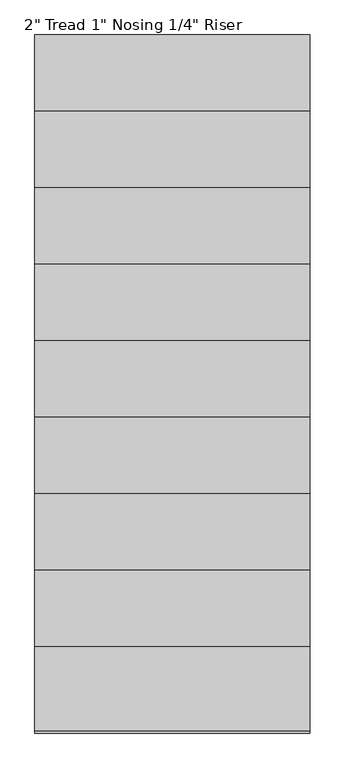
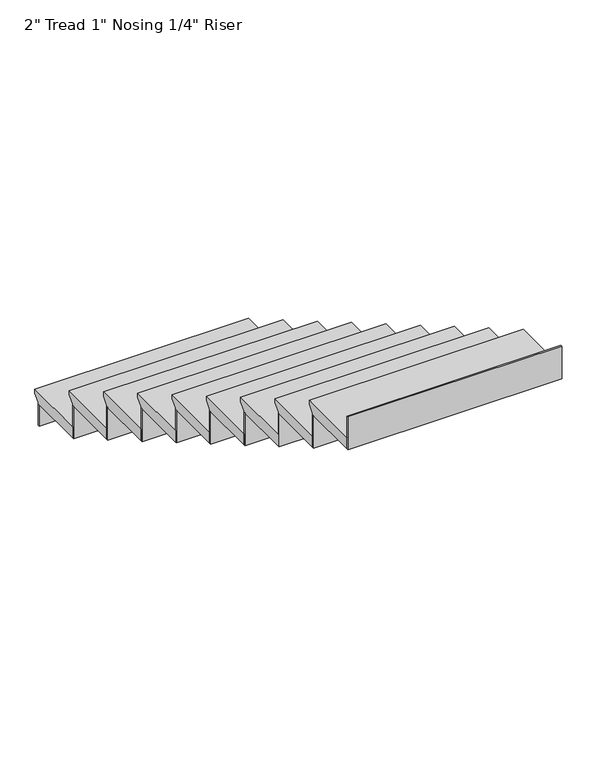
"""IFC4 building model written with IfcOpenShell, lengths in millimetres: stair flight geometry."""

from ifc_helpers import new_model, si_unit, origin, place, context, project, spatial, faceted_brep, source, transform, mapped, element, save


def stair_flight_05c21e37(model_context):
    return source(origin(), model_context, "Body", "Brep", [
        faceted_brep([(-4315.1137331, -4241.0593836, 6472.7714861), (-4315.1137331, -4241.0593836, 6491.8214861), (-3400.7137331, -4241.0593836, 6491.8214861), (-3400.7137331, -4241.0593836, 6472.7714861), (-4315.1137331, -4266.4593836, 6447.3714861), (-3400.7137331, -4266.4593836, 6447.3714861), (-4315.1137331, -4520.4593836, 6491.8214861), (-3400.7137331, -4520.4593836, 6491.8214861), (-3400.7137331, -4266.4593836, 6441.0214861), (-3400.7137331, -4520.4593836, 6441.0214861), (-4315.1137331, -4520.4593836, 6441.0214861), (-4315.1137331, -4266.4593836, 6441.0214861)], [[[0, 1, 2, 3]], [[4, 0, 3, 5]], [[2, 1, 6, 7]], [[8, 9, 10, 11]], [[2, 7, 9, 8, 5, 3]], [[8, 11, 4, 5]], [[6, 1, 0, 4, 11, 10]], [[7, 6, 10, 9]]]),
        faceted_brep([(-4315.1137331, -4266.4593836, 6441.0214861), (-4315.1137331, -4266.4593836, 6343.9725604), (-4315.1137331, -4272.8093836, 6343.9725604), (-4315.1137331, -4272.8093836, 6441.0214861), (-3400.7137331, -4266.4593836, 6441.0214861), (-3400.7137331, -4272.8093836, 6441.0214861), (-3400.7137331, -4272.8093836, 6343.9725604), (-3400.7137331, -4266.4593836, 6343.9725604)], [[[0, 1, 2, 3]], [[4, 5, 6, 7]], [[1, 0, 4, 7]], [[2, 1, 7, 6]], [[3, 2, 6, 5]], [[0, 3, 5, 4]]]),
        faceted_brep([(-4315.1137331, -4520.4593836, 6588.8704118), (-4315.1137331, -4520.4593836, 6441.0214861), (-4315.1137331, -4526.8093836, 6441.0214861), (-4315.1137331, -4526.8093836, 6588.8704118), (-3400.7137331, -4520.4593836, 6588.8704118), (-3400.7137331, -4526.8093836, 6588.8704118), (-3400.7137331, -4526.8093836, 6441.0214861), (-3400.7137331, -4520.4593836, 6441.0214861)], [[[0, 1, 2, 3]], [[4, 5, 6, 7]], [[1, 0, 4, 7]], [[2, 1, 7, 6]], [[3, 2, 6, 5]], [[0, 3, 5, 4]]]),
        faceted_brep([(-3400.7137331, -4495.0593836, 6639.6704118), (-4315.1137331, -4495.0593836, 6639.6704118), (-4315.1137331, -4774.4593836, 6639.6704118), (-3400.7137331, -4774.4593836, 6639.6704118), (-3400.7137331, -4520.4593836, 6588.8704118), (-3400.7137331, -4774.4593836, 6588.8704118), (-4315.1137331, -4774.4593836, 6588.8704118), (-4315.1137331, -4520.4593836, 6588.8704118), (-3400.7137331, -4520.4593836, 6595.2204118), (-3400.7137331, -4495.0593836, 6620.6204118), (-4315.1137331, -4520.4593836, 6595.2204118), (-4315.1137331, -4495.0593836, 6620.6204118)], [[[0, 1, 2, 3]], [[4, 5, 6, 7]], [[0, 3, 5, 4, 8, 9]], [[4, 7, 10, 8]], [[2, 1, 11, 10, 7, 6]], [[3, 2, 6, 5]], [[11, 1, 0, 9]], [[10, 11, 9, 8]]]),
        faceted_brep([(-4315.1137331, -4774.4593836, 6736.7193375), (-4315.1137331, -4774.4593836, 6588.8704118), (-4315.1137331, -4780.8093836, 6588.8704118), (-4315.1137331, -4780.8093836, 6736.7193375), (-3400.7137331, -4774.4593836, 6736.7193375), (-3400.7137331, -4780.8093836, 6736.7193375), (-3400.7137331, -4780.8093836, 6588.8704118), (-3400.7137331, -4774.4593836, 6588.8704118)], [[[0, 1, 2, 3]], [[4, 5, 6, 7]], [[1, 0, 4, 7]], [[2, 1, 7, 6]], [[3, 2, 6, 5]], [[0, 3, 5, 4]]]),
        faceted_brep([(-3400.7137331, -4749.0593836, 6787.5193375), (-4315.1137331, -4749.0593836, 6787.5193375), (-4315.1137331, -5028.4593836, 6787.5193375), (-3400.7137331, -5028.4593836, 6787.5193375), (-3400.7137331, -4774.4593836, 6736.7193375), (-3400.7137331, -5028.4593836, 6736.7193375), (-4315.1137331, -5028.4593836, 6736.7193375), (-4315.1137331, -4774.4593836, 6736.7193375), (-3400.7137331, -4774.4593836, 6743.0693375), (-3400.7137331, -4749.0593836, 6768.4693375), (-4315.1137331, -4774.4593836, 6743.0693375), (-4315.1137331, -4749.0593836, 6768.4693375)], [[[0, 1, 2, 3]], [[4, 5, 6, 7]], [[0, 3, 5, 4, 8, 9]], [[4, 7, 10, 8]], [[2, 1, 11, 10, 7, 6]], [[3, 2, 6, 5]], [[11, 1, 0, 9]], [[10, 11, 9, 8]]]),
        faceted_brep([(-4315.1137331, -5028.4593836, 6884.5682632), (-4315.1137331, -5028.4593836, 6736.7193375), (-4315.1137331, -5034.8093836, 6736.7193375), (-4315.1137331, -5034.8093836, 6884.5682632), (-3400.7137331, -5028.4593836, 6884.5682632), (-3400.7137331, -5034.8093836, 6884.5682632), (-3400.7137331, -5034.8093836, 6736.7193375), (-3400.7137331, -5028.4593836, 6736.7193375)], [[[0, 1, 2, 3]], [[4, 5, 6, 7]], [[1, 0, 4, 7]], [[2, 1, 7, 6]], [[3, 2, 6, 5]], [[0, 3, 5, 4]]]),
        faceted_brep([(-3400.7137331, -5003.0593836, 6935.3682632), (-4315.1137331, -5003.0593836, 6935.3682632), (-4315.1137331, -5282.4593836, 6935.3682632), (-3400.7137331, -5282.4593836, 6935.3682632), (-3400.7137331, -5028.4593836, 6884.5682632), (-3400.7137331, -5282.4593836, 6884.5682632), (-4315.1137331, -5282.4593836, 6884.5682632), (-4315.1137331, -5028.4593836, 6884.5682632), (-3400.7137331, -5028.4593836, 6890.9182632), (-3400.7137331, -5003.0593836, 6916.3182632), (-4315.1137331, -5028.4593836, 6890.9182632), (-4315.1137331, -5003.0593836, 6916.3182632)], [[[0, 1, 2, 3]], [[4, 5, 6, 7]], [[0, 3, 5, 4, 8, 9]], [[4, 7, 10, 8]], [[2, 1, 11, 10, 7, 6]], [[3, 2, 6, 5]], [[11, 1, 0, 9]], [[10, 11, 9, 8]]]),
        faceted_brep([(-4315.1137331, -5282.4593836, 7032.4171889), (-4315.1137331, -5282.4593836, 6884.5682632), (-4315.1137331, -5288.8093836, 6884.5682632), (-4315.1137331, -5288.8093836, 7032.4171889), (-3400.7137331, -5282.4593836, 7032.4171889), (-3400.7137331, -5288.8093836, 7032.4171889), (-3400.7137331, -5288.8093836, 6884.5682632), (-3400.7137331, -5282.4593836, 6884.5682632)], [[[0, 1, 2, 3]], [[4, 5, 6, 7]], [[1, 0, 4, 7]], [[2, 1, 7, 6]], [[3, 2, 6, 5]], [[0, 3, 5, 4]]]),
        faceted_brep([(-3400.7137331, -5257.0593836, 7083.2171889), (-4315.1137331, -5257.0593836, 7083.2171889), (-4315.1137331, -5536.4593836, 7083.2171889), (-3400.7137331, -5536.4593836, 7083.2171889), (-3400.7137331, -5282.4593836, 7032.4171889), (-3400.7137331, -5536.4593836, 7032.4171889), (-4315.1137331, -5536.4593836, 7032.4171889), (-4315.1137331, -5282.4593836, 7032.4171889), (-3400.7137331, -5282.4593836, 7038.7671889), (-3400.7137331, -5257.0593836, 7064.1671889), (-4315.1137331, -5282.4593836, 7038.7671889), (-4315.1137331, -5257.0593836, 7064.1671889)], [[[0, 1, 2, 3]], [[4, 5, 6, 7]], [[0, 3, 5, 4, 8, 9]], [[4, 7, 10, 8]], [[2, 1, 11, 10, 7, 6]], [[3, 2, 6, 5]], [[11, 1, 0, 9]], [[10, 11, 9, 8]]]),
        faceted_brep([(-4315.1137331, -5536.4593836, 7180.2661146), (-4315.1137331, -5536.4593836, 7032.4171889), (-4315.1137331, -5542.8093836, 7032.4171889), (-4315.1137331, -5542.8093836, 7180.2661146), (-3400.7137331, -5536.4593836, 7180.2661146), (-3400.7137331, -5542.8093836, 7180.2661146), (-3400.7137331, -5542.8093836, 7032.4171889), (-3400.7137331, -5536.4593836, 7032.4171889)], [[[0, 1, 2, 3]], [[4, 5, 6, 7]], [[1, 0, 4, 7]], [[2, 1, 7, 6]], [[3, 2, 6, 5]], [[0, 3, 5, 4]]]),
        faceted_brep([(-3400.7137331, -5511.0593836, 7231.0661146), (-4315.1137331, -5511.0593836, 7231.0661146), (-4315.1137331, -5790.4593836, 7231.0661146), (-3400.7137331, -5790.4593836, 7231.0661146), (-3400.7137331, -5536.4593836, 7180.2661146), (-3400.7137331, -5790.4593836, 7180.2661146), (-4315.1137331, -5790.4593836, 7180.2661146), (-4315.1137331, -5536.4593836, 7180.2661146), (-3400.7137331, -5536.4593836, 7186.6161146), (-3400.7137331, -5511.0593836, 7212.0161146), (-4315.1137331, -5536.4593836, 7186.6161146), (-4315.1137331, -5511.0593836, 7212.0161146)], [[[0, 1, 2, 3]], [[4, 5, 6, 7]], [[0, 3, 5, 4, 8, 9]], [[4, 7, 10, 8]], [[2, 1, 11, 10, 7, 6]], [[3, 2, 6, 5]], [[11, 1, 0, 9]], [[10, 11, 9, 8]]]),
        faceted_brep([(-4315.1137331, -5790.4593836, 7328.1150403), (-4315.1137331, -5790.4593836, 7180.2661146), (-4315.1137331, -5796.8093836, 7180.2661146), (-4315.1137331, -5796.8093836, 7328.1150403), (-3400.7137331, -5790.4593836, 7328.1150403), (-3400.7137331, -5796.8093836, 7328.1150403), (-3400.7137331, -5796.8093836, 7180.2661146), (-3400.7137331, -5790.4593836, 7180.2661146)], [[[0, 1, 2, 3]], [[4, 5, 6, 7]], [[1, 0, 4, 7]], [[2, 1, 7, 6]], [[3, 2, 6, 5]], [[0, 3, 5, 4]]]),
        faceted_brep([(-3400.7137331, -5765.0593836, 7378.9150403), (-4315.1137331, -5765.0593836, 7378.9150403), (-4315.1137331, -6044.4593836, 7378.9150403), (-3400.7137331, -6044.4593836, 7378.9150403), (-3400.7137331, -5790.4593836, 7328.1150403), (-3400.7137331, -6044.4593836, 7328.1150403), (-4315.1137331, -6044.4593836, 7328.1150403), (-4315.1137331, -5790.4593836, 7328.1150403), (-3400.7137331, -5790.4593836, 7334.4650403), (-3400.7137331, -5765.0593836, 7359.8650403), (-4315.1137331, -5790.4593836, 7334.4650403), (-4315.1137331, -5765.0593836, 7359.8650403)], [[[0, 1, 2, 3]], [[4, 5, 6, 7]], [[0, 3, 5, 4, 8, 9]], [[4, 7, 10, 8]], [[2, 1, 11, 10, 7, 6]], [[3, 2, 6, 5]], [[11, 1, 0, 9]], [[10, 11, 9, 8]]]),
        faceted_brep([(-4315.1137331, -6044.4593836, 7475.963966), (-4315.1137331, -6044.4593836, 7328.1150403), (-4315.1137331, -6050.8093836, 7328.1150403), (-4315.1137331, -6050.8093836, 7475.963966), (-3400.7137331, -6044.4593836, 7475.963966), (-3400.7137331, -6050.8093836, 7475.963966), (-3400.7137331, -6050.8093836, 7328.1150403), (-3400.7137331, -6044.4593836, 7328.1150403)], [[[0, 1, 2, 3]], [[4, 5, 6, 7]], [[1, 0, 4, 7]], [[2, 1, 7, 6]], [[3, 2, 6, 5]], [[0, 3, 5, 4]]]),
        faceted_brep([(-3400.7137331, -6019.0593836, 7526.763966), (-4315.1137331, -6019.0593836, 7526.763966), (-4315.1137331, -6298.4593836, 7526.763966), (-3400.7137331, -6298.4593836, 7526.763966), (-3400.7137331, -6044.4593836, 7475.963966), (-3400.7137331, -6298.4593836, 7475.963966), (-4315.1137331, -6298.4593836, 7475.963966), (-4315.1137331, -6044.4593836, 7475.963966), (-3400.7137331, -6044.4593836, 7482.313966), (-3400.7137331, -6019.0593836, 7507.713966), (-4315.1137331, -6044.4593836, 7482.313966), (-4315.1137331, -6019.0593836, 7507.713966)], [[[0, 1, 2, 3]], [[4, 5, 6, 7]], [[0, 3, 5, 4, 8, 9]], [[4, 7, 10, 8]], [[2, 1, 11, 10, 7, 6]], [[3, 2, 6, 5]], [[11, 1, 0, 9]], [[10, 11, 9, 8]]]),
        faceted_brep([(-4315.1137331, -6552.4593836, 7771.6618174), (-4315.1137331, -6552.4593836, 7623.8128917), (-4315.1137331, -6558.8093836, 7623.8128917), (-4315.1137331, -6558.8093836, 7771.6618174), (-3400.7137331, -6552.4593836, 7771.6618174), (-3400.7137331, -6558.8093836, 7771.6618174), (-3400.7137331, -6558.8093836, 7623.8128917), (-3400.7137331, -6552.4593836, 7623.8128917)], [[[0, 1, 2, 3]], [[4, 5, 6, 7]], [[1, 0, 4, 7]], [[2, 1, 7, 6]], [[3, 2, 6, 5]], [[0, 3, 5, 4]]]),
        faceted_brep([(-4315.1137331, -6298.4593836, 7623.8128917), (-4315.1137331, -6298.4593836, 7475.963966), (-4315.1137331, -6304.8093836, 7475.963966), (-4315.1137331, -6304.8093836, 7623.8128917), (-3400.7137331, -6298.4593836, 7623.8128917), (-3400.7137331, -6304.8093836, 7623.8128917), (-3400.7137331, -6304.8093836, 7475.963966), (-3400.7137331, -6298.4593836, 7475.963966)], [[[0, 1, 2, 3]], [[4, 5, 6, 7]], [[1, 0, 4, 7]], [[2, 1, 7, 6]], [[3, 2, 6, 5]], [[0, 3, 5, 4]]]),
        faceted_brep([(-3400.7137331, -6552.4593836, 7674.6128917), (-3400.7137331, -6527.0593836, 7674.6128917), (-3400.7137331, -6273.0593836, 7674.6128917), (-4315.1137331, -6273.0593836, 7674.6128917), (-4315.1137331, -6552.4593836, 7674.6128917), (-3400.7137331, -6527.0593836, 7623.8128917), (-3400.7137331, -6552.4593836, 7623.8128917), (-4315.1137331, -6552.4593836, 7623.8128917), (-4315.1137331, -6298.4593836, 7623.8128917), (-3400.7137331, -6298.4593836, 7623.8128917), (-3400.7137331, -6298.4593836, 7630.1628917), (-3400.7137331, -6273.0593836, 7655.5628917), (-4315.1137331, -6298.4593836, 7630.1628917), (-4315.1137331, -6273.0593836, 7655.5628917)], [[[0, 1, 2, 3, 4]], [[5, 6, 7, 8, 9]], [[1, 0, 6, 5]], [[2, 1, 5, 9, 10, 11]], [[9, 8, 12, 10]], [[4, 3, 13, 12, 8, 7]], [[0, 4, 7, 6]], [[13, 3, 2, 11]], [[12, 13, 11, 10]]]),
    ])


if __name__ == "__main__":
    model = new_model("IFC4")
    model_context = context("Model", 3, world=origin())
    ifc_project = project(units=[si_unit("LENGTHUNIT", "METRE", prefix="MILLI")], contexts=[model_context])
    site = spatial("IfcSite", under=ifc_project)
    building = spatial("IfcBuilding", under=site)
    placement = place(None, origin())
    stair_flight_shape = stair_flight_05c21e37(model_context)
    element("IfcStairFlight", 1, ObjectType="2\" Tread 1\" Nosing 1/4\" Riser", at=placement, inside=building, context=model_context, shape_type="MappedRepresentation", body=[
        mapped(stair_flight_shape, transform((0.0, 0.0, 0.0), x_axis=(1.0, 0.0, 0.0), y_axis=(0.0, 1.0, 0.0), z_axis=(0.0, 0.0, 1.0))),
    ])
    save(model, "model.ifc")
